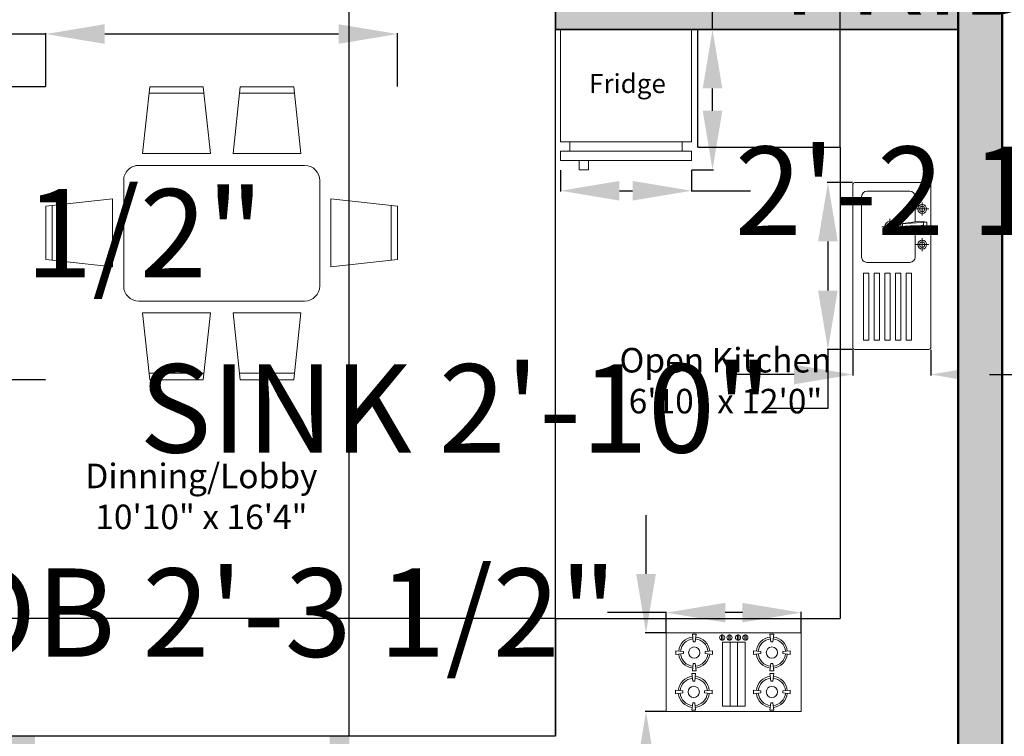
# Model space of a CAD drawing. Units: inches. Extents: x 2796 to 3603, y 978 to 1787.
# Tile 10 of 15: x 3224 to 3425, y 1312 to 1458. Entities that reach past the tile are written whole.
import ezdxf

# ---------------------------------------------------------------- set-up
doc = ezdxf.new("R2010")
doc.units = ezdxf.units.IN
for name, color, linetype, lineweight in [('A-ANNO-DIMS', 7, 'Continuous', 18), ('A-ANNO-TEXT', 7, 'Continuous', 18), ('A-AREA-IDEN', 7, 'Continuous', 18), ('A-EQPM', 3, 'Continuous', 18), ('A-FLOR-FIXT', 8, 'Continuous', 18), ('A-WALL-EXTR-PATT', 1, 'Continuous', 13), ('A-WALL-INTR-PATT', 5, 'Continuous', 13), ('Furniture', 2, 'Continuous', 18), ('Inner Wall', 5, 'Continuous', 35), ('Kitchen', 3, 'Continuous', 25), ('Outer Wall', 1, 'Continuous', 50)]:
    doc.layers.add(name, color=color, linetype=linetype, lineweight=lineweight)
doc.styles.get("Standard").update_dxf_attribs({"font": 'arial.ttf'})
doc.dimstyles.get("Standard").update_dxf_attribs({"dimtxt": 18, "dimasz": 12, "dimexe": 0.18, "dimexo": 0.0625, "dimgap": 0.09, "dimtad": 0, "dimtih": 1, "dimtoh": 1, "dimdec": 0, "dimzin": 0, "dimdsep": 46, "dimlunit": 3, "dimtxsty": 'Standard', "dimcen": 0.09, "dimadec": 0, "dimazin": 0, "dimtfac": 1, "dimtdec": 0, "dimtofl": 0, "dimtmove": 0, "dimatfit": 3, "dimfxl": 1, "dimtolj": 1, "dimtzin": 0, "dimarcsym": 0})

# ---------------------------------------------------------------- blocks, each defined once
blk = doc.blocks.new('A$C6D1B16CF')
for p, q in [((0.6411, 1.5), (0.6886, 1.9429)), ((0.684, 1.9), (1.0481, 1.9)), ((0.6886, 1.9429), (1.0435, 1.9429)), ((1.0435, 1.9429), (1.091, 1.5)), ((1.2411, 1.5), (1.2886, 1.9429)), ((1.284, 1.9), (1.6481, 1.9)), ((1.2886, 1.9429), (1.6435, 1.9429)), ((1.6435, 1.9429), (1.691, 1.5)), ((1.091, 1.5), (0.6411, 1.5)), ((1.691, 1.5), (1.2411, 1.5)), ((0.6161, 1.4214), (1.7161, 1.4214)), ((0.5161, 0.6214), (0.5161, 1.3214)), ((1.8161, 1.3214), (1.8161, 0.6214)), ((0, 1.1464), (0.4429, 1.1939)), ((0.4429, 1.1939), (0.4429, 0.744)), ((2.3321, 1.1464), (1.8892, 1.1939)), ((1.8892, 1.1939), (1.8892, 0.744)), ((0, 0.7916), (0, 1.1464)), ((0.0429, 0.787), (0.0429, 1.151)), ((2.2892, 0.787), (2.2892, 1.151)), ((2.3321, 0.7916), (2.3321, 1.1464)), ((0.4429, 0.744), (0, 0.7916)), ((1.8892, 0.744), (2.3321, 0.7916)), ((1.7161, 0.5214), (0.6161, 0.5214)), ((1.091, 0.4429), (0.6411, 0.4429)), ((0.6411, 0.4429), (0.6886, 0)), ((1.0435, 0), (1.091, 0.4429)), ((1.691, 0.4429), (1.2411, 0.4429)), ((1.2411, 0.4429), (1.2886, 0)), ((1.6435, 0), (1.691, 0.4429)), ((0.684, 0.0429), (1.0481, 0.0429)), ((0.6886, 0), (1.0435, 0)), ((1.284, 0.0429), (1.6481, 0.0429)), ((1.2886, 0), (1.6435, 0))]:
    blk.add_line(p, q)
for centre, start, end in [((0.6161, 1.3214), 90, 180), ((1.7161, 1.3214), 0, 90), ((0.6161, 0.6214), 180, 270), ((1.7161, 0.6214), 270, 0)]:
    blk.add_arc(centre, 0.1, start, end)
blk = doc.blocks.new('A$C57CF26DA')
for p, q in [((0, 0), (0, 420)), ((720, 420), (0, 420)), ((166.9, 413), (146.9, 413)), ((146.9, 413), (151.9, 373)), ((151.9, 373), (161.9, 373)), ((161.9, 373), (166.9, 413)), ((300, 390.9), (300, 49.1)), ((300, 390.9), (420, 390.9)), ((340, 390.9), (340, 49.1)), ((380, 390.9), (380, 49.1)), ((420, 390.9), (420, 49.1)), ((583.6, 413), (563.6, 413)), ((563.6, 413), (568.6, 373)), ((568.6, 373), (578.6, 373)), ((578.6, 373), (583.6, 413)), ((720, 0), (720, 420)), ((98.9, 320), (58.9, 325)), ((58.9, 325), (58.9, 305)), ((98.9, 310), (98.9, 320)), ((254.8, 325), (214.8, 320)), ((214.8, 320), (214.8, 310)), ((254.8, 305), (254.8, 325)), ((515.6, 320), (475.6, 325)), ((475.6, 325), (475.6, 305)), ((515.6, 310), (515.6, 320)), ((671.6, 325), (631.6, 320)), ((631.6, 320), (631.6, 310)), ((671.6, 305), (671.6, 325)), ((58.9, 305), (98.9, 310)), ((214.8, 310), (254.8, 305)), ((475.6, 305), (515.6, 310)), ((631.6, 310), (671.6, 305)), ((151.9, 257), (146.9, 217)), ((146.9, 217), (166.9, 217)), ((161.9, 257), (151.9, 257)), ((166.9, 217), (161.9, 257)), ((568.6, 257), (563.6, 217)), ((563.6, 217), (583.6, 217)), ((578.6, 257), (568.6, 257)), ((583.6, 217), (578.6, 257)), ((166.9, 203), (146.9, 203)), ((146.9, 203), (151.9, 163)), ((151.9, 163), (161.9, 163)), ((161.9, 163), (166.9, 203)), ((581.1, 203), (561.1, 203)), ((561.1, 203), (566.1, 163)), ((566.1, 163), (576.1, 163)), ((576.1, 163), (581.1, 203)), ((98.9, 110), (58.9, 115)), ((58.9, 115), (58.9, 95)), ((98.9, 100), (98.9, 110)), ((254.8, 115), (214.8, 110)), ((214.8, 110), (214.8, 100)), ((254.8, 95), (254.8, 115)), ((513.1, 110), (473.1, 115)), ((473.1, 115), (473.1, 95)), ((513.1, 100), (513.1, 110)), ((669, 115), (629, 110)), ((629, 110), (629, 100)), ((669, 95), (669, 115)), ((58.9, 95), (98.9, 100)), ((214.8, 100), (254.8, 95)), ((473.1, 95), (513.1, 100)), ((629, 100), (669, 95)), ((151.9, 47), (146.9, 7)), ((146.9, 7), (166.9, 7)), ((161.9, 47), (151.9, 47)), ((166.9, 7), (161.9, 47)), ((301.5, 38.7), (294.7, 38.7)), ((294.7, 38.7), (294.7, 11.3)), ((294.7, 11.3), (301.5, 11.3)), ((420, 49.1), (300, 49.1)), ((301.5, 11.3), (301.5, 38.7)), ((340.5, 38.7), (333.7, 38.7)), ((333.7, 38.7), (333.7, 11.3)), ((333.7, 11.3), (340.5, 11.3)), ((340.5, 11.3), (340.5, 38.7)), ((379.7, 11.3), (379.7, 38.7)), ((379.7, 38.7), (386.5, 38.7)), ((386.5, 11.3), (379.7, 11.3)), ((386.5, 38.7), (386.5, 11.3)), ((418.7, 11.3), (418.7, 38.7)), ((418.7, 38.7), (425.5, 38.7)), ((425.5, 11.3), (418.7, 11.3)), ((425.5, 38.7), (425.5, 11.3)), ((566.1, 47), (561.1, 7)), ((561.1, 7), (581.1, 7)), ((576.1, 47), (566.1, 47)), ((581.1, 7), (576.1, 47)), ((720, 0), (0, 0))]:
    blk.add_line(p, q)
for centre in [(156.9, 315), (573.6, 315), (156.9, 105), (571.1, 105)]:
    blk.add_circle(centre, 30)
for centre, radius, start, end in [((156.9, 315), 83, 95.5849, 174.4151), ((156.9, 315), 73, 95.3738, 174.6262), ((156.9, 315), 73, 5.3738, 84.6262), ((156.9, 315), 83, 5.5849, 84.4151), ((573.6, 315), 83, 95.5849, 174.4151), ((573.6, 315), 73, 95.3738, 174.6262), ((573.6, 315), 73, 5.3738, 84.6262), ((573.6, 315), 83, 5.5849, 84.4151), ((156.9, 315), 83, 185.5849, 264.4151), ((156.9, 315), 73, 185.3738, 264.6262), ((156.9, 315), 73, 275.3738, 354.6262), ((156.9, 315), 83, 275.5849, 354.4151), ((573.6, 315), 83, 185.5849, 264.4151), ((573.6, 315), 73, 185.3738, 264.6262), ((573.6, 315), 73, 275.3738, 354.6262), ((573.6, 315), 83, 275.5849, 354.4151), ((156.9, 105), 83, 95.5849, 174.4151), ((156.9, 105), 73, 95.3738, 174.6262), ((156.9, 105), 73, 5.3738, 84.6262), ((156.9, 105), 83, 5.5849, 84.4151), ((571.1, 105), 83, 95.5849, 174.4151), ((571.1, 105), 73, 95.3738, 174.6262), ((571.1, 105), 73, 5.3738, 84.6262), ((571.1, 105), 83, 5.5849, 84.4151), ((156.9, 105), 83, 185.5849, 264.4151), ((156.9, 105), 73, 185.3738, 264.6262), ((156.9, 105), 73, 275.3738, 354.6262), ((156.9, 105), 83, 275.5849, 354.4151), ((571.1, 105), 83, 185.5849, 264.4151), ((571.1, 105), 73, 185.3738, 264.6262), ((571.1, 105), 73, 275.3738, 354.6262), ((571.1, 105), 83, 275.5849, 354.4151), ((298.1, 25), 13.7, 104.4775, 255.5225), ((298.1, 25), 13.7, 284.4775, 75.5225), ((337.1, 25), 13.7, 104.4775, 255.5225), ((337.1, 25), 13.7, 284.4775, 75.5225), ((383.1, 25), 13.7, 104.4775, 255.5225), ((383.1, 25), 13.7, 284.4775, 75.5225), ((422.1, 25), 13.7, 104.4775, 255.5225), ((422.1, 25), 13.7, 284.4775, 75.5225)]:
    blk.add_arc(centre, radius, start, end)
blk = doc.blocks.new('A$C7C492201')
for p, q in [((0, 10), (0, 426.6)), ((10, 436.6), (927.3, 436.6)), ((111.9, 388.7), (185, 388.7)), ((148.5, 425.2), (148.5, 352.2)), ((223.5, 415), (217, 376.2)), ((223.5, 415), (231.8, 268.5)), ((223.5, 415), (248.5, 415)), ((224.6, 395.4), (248.5, 395.4)), ((273.5, 415), (248.5, 415)), ((272.3, 395.4), (248.5, 395.4)), ((273.5, 415), (265.2, 268.5)), ((273.5, 415), (279.9, 376.2)), ((311.9, 388.7), (385, 388.7)), ((348.5, 425.2), (348.5, 352.2)), ((937.3, 10), (937.3, 426.6)), ((220.8, 348.8), (78.5, 348.8)), ((217, 376.2), (231.8, 268.5)), ((279.9, 376.2), (265.2, 268.5)), ((418.5, 348.8), (276.2, 348.8)), ((48.5, 318.8), (48.5, 78.8)), ((231.3, 278.6), (248.5, 278.6)), ((265.6, 278.6), (248.5, 278.6)), ((448.5, 318.8), (448.5, 78.8)), ((509.1, 328.4), (509.1, 298.4)), ((509.1, 328.4), (885, 328.4)), ((509.1, 298.4), (885, 298.4)), ((885, 328.4), (885, 298.4)), ((231.8, 268.5), (248.5, 268.5)), ((265.2, 268.5), (248.5, 268.5)), ((248.5, 252.8), (248.5, 162.6)), ((509.1, 268.4), (509.1, 238.4)), ((509.1, 268.4), (885, 268.4)), ((509.1, 238.4), (885, 238.4)), ((885, 268.4), (885, 238.4)), ((203.4, 207.7), (293.5, 207.7)), ((509.1, 208.4), (885, 208.4)), ((509.1, 208.4), (509.1, 178.4)), ((509.1, 178.4), (885, 178.4)), ((885, 208.4), (885, 178.4)), ((509.1, 148.4), (509.1, 118.4)), ((509.1, 148.4), (885, 148.4)), ((509.1, 118.4), (885, 118.4)), ((885, 148.4), (885, 118.4)), ((509.1, 88.4), (509.1, 58.4)), ((509.1, 88.4), (885, 88.4)), ((509.1, 58.4), (885, 58.4)), ((885, 88.4), (885, 58.4)), ((927.3, 0), (10, 0)), ((418.5, 48.8), (78.5, 48.8))]:
    blk.add_line(p, q)
for centre, radius in [((148.5, 388.7), 25), ((148.5, 388.7), 15), ((348.5, 388.7), 25), ((348.5, 388.7), 15), ((248.5, 207.7), 30), ((248.5, 207.7), 20)]:
    blk.add_circle(centre, radius)
for centre, radius, start, end in [((10, 426.6), 10, 90, 180), ((247.3, 388), 7.19, 80.5252, 279.4748), ((249.6, 388), 7.19, 260.5252, 99.4748), ((927.3, 426.6), 10, 0, 90), ((78.5, 318.8), 30, 90, 180), ((418.5, 318.8), 30, 0, 90), ((78.5, 78.8), 30, 180, 270), ((418.5, 78.8), 30, 270, 0), ((10, 10), 10, 180, 270), ((927.3, 10), 10, 270, 0)]:
    blk.add_arc(centre, radius, start, end)
blk = doc.blocks.new('REFRI-00')
for points in [[(-0.35, 0.35), (-0.35, -0.25), (0.35, -0.25), (0.35, 0.35), (-0.35, 0.35)], [(-0.3, -0.3), (-0.3, -0.25)], [(0.3, -0.3), (0.3, -0.25)], [(-0.35, -0.3), (-0.35, -0.35), (0.35, -0.35), (0.35, -0.3), (-0.35, -0.3)], [(-0.25, -0.35), (-0.25, -0.4), (-0.2, -0.4), (-0.2, -0.35)]]:
    blk.add_lwpolyline(points)
blk = doc.blocks.new('*D32')
at = {"layer": 'A-ANNO-DIMS', "color": 0, "lineweight": -2, "transparency": 16777216}
for p, q in [((3229.46, 1454.75), (3217.46, 1454.75)), ((3229.46, 1444.07), (3229.46, 1454.93)), ((3289.09, 1454.75), (3241.46, 1454.75)), ((3301.09, 1444.07), (3301.09, 1454.93))]:
    blk.add_line(p, q, dxfattribs=at)
at = {"layer": 'A-ANNO-DIMS', "color": 0, "transparency": 16777216}
for points in [[(3241.46, 1456.75), (3241.46, 1452.75), (3229.46, 1454.75)], [(3289.09, 1456.75), (3289.09, 1452.75), (3301.09, 1454.75)]]:
    blk.add_solid(points, dxfattribs=at)
at = {"layer": 'Defpoints', "color": 0, "transparency": 16777216}
for p in [(3229.46, 1454.75), (3229.46, 1444.01), (3301.09, 1444.01)]:
    blk.add_point(p, dxfattribs=at)
at = {"layer": 'A-ANNO-DIMS', "color": 0, "transparency": 16777216, "insert": (3090.48, 1454.75), "char_height": 18, "attachment_point": 5}
blk.add_mtext('\\A1;DINING SET 5\'-11 1/2"', dxfattribs=at)
blk = doc.blocks.new('*D33')
at = {"layer": 'A-ANNO-DIMS', "color": 0, "lineweight": -2, "transparency": 16777216}
for p, q in [((3229.39, 1444.01), (3218.53, 1444.01)), ((3218.71, 1432.01), (3218.71, 1423.57)), ((3218.71, 1396.33), (3218.71, 1404.77)), ((3229.39, 1384.33), (3218.53, 1384.33))]:
    blk.add_line(p, q, dxfattribs=at)
at = {"layer": 'A-ANNO-DIMS', "color": 0, "transparency": 16777216}
for points in [[(3216.71, 1432.01), (3220.71, 1432.01), (3218.71, 1444.01)], [(3216.71, 1396.33), (3220.71, 1396.33), (3218.71, 1384.33)]]:
    blk.add_solid(points, dxfattribs=at)
at = {"layer": 'Defpoints', "color": 0, "transparency": 16777216}
for p in [(3229.46, 1444.01), (3218.71, 1384.33), (3229.46, 1384.33)]:
    blk.add_point(p, dxfattribs=at)
at = {"layer": 'A-ANNO-DIMS', "color": 0, "transparency": 16777216, "insert": (3218.71, 1414.17), "char_height": 18, "attachment_point": 5}
blk.add_mtext('\\A1;4\'-11 1/2"', dxfattribs=at)
blk = doc.blocks.new('*D34')
at = {"layer": 'A-ANNO-DIMS', "color": 0, "lineweight": -2, "transparency": 16777216}
for p, q in [((3355.83, 1336.87), (3343.83, 1336.87)), ((3355.83, 1332.81), (3355.83, 1337.05)), ((3371.32, 1336.87), (3367.83, 1336.87)), ((3383.32, 1332.81), (3383.32, 1337.05))]:
    blk.add_line(p, q, dxfattribs=at)
at = {"layer": 'A-ANNO-DIMS', "color": 0, "transparency": 16777216}
for points in [[(3367.83, 1338.87), (3367.83, 1334.87), (3355.83, 1336.87)], [(3371.32, 1338.87), (3371.32, 1334.87), (3383.32, 1336.87)]]:
    blk.add_solid(points, dxfattribs=at)
at = {"layer": 'Defpoints', "color": 0, "transparency": 16777216}
for p in [(3355.83, 1336.87), (3355.83, 1332.75), (3383.32, 1332.75)]:
    blk.add_point(p, dxfattribs=at)
at = {"layer": 'A-ANNO-DIMS', "color": 0, "transparency": 16777216, "insert": (3268.59, 1336.87), "char_height": 18, "attachment_point": 5}
blk.add_mtext('\\A1;HOB 2\'-3 1/2"', dxfattribs=at)
blk = doc.blocks.new('*D35')
at = {"layer": 'A-ANNO-DIMS', "color": 0, "lineweight": -2, "transparency": 16777216}
for p, q in [((3351.71, 1344.75), (3351.71, 1356.75)), ((3355.77, 1332.75), (3351.53, 1332.75)), ((3355.77, 1316.72), (3351.53, 1316.72)), ((3351.71, 1304.72), (3351.71, 1292.72)), ((3351.71, 1292.72), (3339.71, 1292.72))]:
    blk.add_line(p, q, dxfattribs=at)
at = {"layer": 'A-ANNO-DIMS', "color": 0, "transparency": 16777216}
for points in [[(3349.71, 1344.75), (3353.71, 1344.75), (3351.71, 1332.75)], [(3349.71, 1304.72), (3353.71, 1304.72), (3351.71, 1316.72)]]:
    blk.add_solid(points, dxfattribs=at)
at = {"layer": 'Defpoints', "color": 0, "transparency": 16777216}
for p in [(3355.83, 1332.75), (3351.71, 1316.72), (3355.83, 1316.72)]:
    blk.add_point(p, dxfattribs=at)
at = {"layer": 'A-ANNO-DIMS', "color": 0, "transparency": 16777216, "insert": (3316.54, 1292.72), "char_height": 18, "attachment_point": 5}
blk.add_mtext('\\A1;1\'-4"', dxfattribs=at)
blk = doc.blocks.new('*D36')
at = {"layer": 'A-ANNO-DIMS', "color": 0, "lineweight": -2, "transparency": 16777216}
for p, q in [((3393.79, 1424.5), (3388.57, 1424.5)), ((3388.75, 1412.5), (3388.75, 1402.49)), ((3393.79, 1390.49), (3388.57, 1390.49)), ((3388.75, 1390.49), (3388.75, 1378.49)), ((3388.75, 1378.49), (3376.75, 1378.49))]:
    blk.add_line(p, q, dxfattribs=at)
at = {"layer": 'A-ANNO-DIMS', "color": 0, "transparency": 16777216}
for points in [[(3386.75, 1412.5), (3390.75, 1412.5), (3388.75, 1424.5)], [(3386.75, 1402.49), (3390.75, 1402.49), (3388.75, 1390.49)]]:
    blk.add_solid(points, dxfattribs=at)
at = {"layer": 'Defpoints', "color": 0, "transparency": 16777216}
for p in [(3393.85, 1424.5), (3388.75, 1390.49), (3393.85, 1390.49)]:
    blk.add_point(p, dxfattribs=at)
at = {"layer": 'A-ANNO-DIMS', "color": 0, "transparency": 16777216, "insert": (3312.95, 1378.49), "char_height": 18, "attachment_point": 5}
blk.add_mtext('\\A1;SINK 2\'-10"', dxfattribs=at)
blk = doc.blocks.new('*D37')
at = {"layer": 'A-ANNO-DIMS', "color": 0, "lineweight": -2, "transparency": 16777216}
for p, q in [((3393.85, 1390.43), (3393.85, 1385.21)), ((3409.69, 1390.43), (3409.69, 1385.21)), ((3381.85, 1385.39), (3369.85, 1385.39)), ((3421.69, 1385.39), (3433.69, 1385.39))]:
    blk.add_line(p, q, dxfattribs=at)
at = {"layer": 'A-ANNO-DIMS', "color": 0, "transparency": 16777216}
for points in [[(3381.85, 1387.39), (3381.85, 1383.39), (3393.85, 1385.39)], [(3421.69, 1387.39), (3421.69, 1383.39), (3409.69, 1385.39)]]:
    blk.add_solid(points, dxfattribs=at)
at = {"layer": 'Defpoints', "color": 0, "transparency": 16777216}
for p in [(3393.85, 1390.49), (3409.69, 1390.49), (3409.69, 1385.39)]:
    blk.add_point(p, dxfattribs=at)
at = {"layer": 'A-ANNO-DIMS', "color": 0, "transparency": 16777216, "insert": (3456.86, 1385.39), "char_height": 18, "attachment_point": 5}
blk.add_mtext('\\A1;1\'-4"', dxfattribs=at)
blk = doc.blocks.new('*D38')
at = {"layer": 'A-ANNO-DIMS', "color": 0, "lineweight": -2, "transparency": 16777216}
for p, q in [((3365.25, 1455.68), (3365.25, 1467.68)), ((3365.25, 1467.68), (3377.25, 1467.68)), ((3361.02, 1455.68), (3365.43, 1455.68)), ((3365.25, 1439.11), (3365.25, 1443.68)), ((3361.02, 1427.11), (3365.43, 1427.11))]:
    blk.add_line(p, q, dxfattribs=at)
at = {"layer": 'A-ANNO-DIMS', "color": 0, "transparency": 16777216}
for points in [[(3363.25, 1443.68), (3367.25, 1443.68), (3365.25, 1455.68)], [(3363.25, 1439.11), (3367.25, 1439.11), (3365.25, 1427.11)]]:
    blk.add_solid(points, dxfattribs=at)
at = {"layer": 'Defpoints', "color": 0, "transparency": 16777216}
for p in [(3360.96, 1455.68), (3365.25, 1455.68), (3360.96, 1427.11)]:
    blk.add_point(p, dxfattribs=at)
at = {"layer": 'A-ANNO-DIMS', "color": 0, "transparency": 16777216, "insert": (3472.71, 1467.68), "char_height": 18, "attachment_point": 5}
blk.add_mtext('\\A1;FRIDGE 2\'-4 1/2"', dxfattribs=at)
blk = doc.blocks.new('*D39')
at = {"layer": 'A-ANNO-DIMS', "color": 0, "lineweight": -2, "transparency": 16777216}
for p, q in [((3334.3, 1427.04), (3334.3, 1422.64)), ((3360.96, 1427.04), (3360.96, 1422.64)), ((3346.3, 1422.82), (3348.96, 1422.82)), ((3360.96, 1422.82), (3372.96, 1422.82))]:
    blk.add_line(p, q, dxfattribs=at)
at = {"layer": 'A-ANNO-DIMS', "color": 0, "transparency": 16777216}
for points in [[(3346.3, 1424.82), (3346.3, 1420.82), (3334.3, 1422.82)], [(3348.96, 1424.82), (3348.96, 1420.82), (3360.96, 1422.82)]]:
    blk.add_solid(points, dxfattribs=at)
at = {"layer": 'Defpoints', "color": 0, "transparency": 16777216}
for p in [(3334.3, 1427.11), (3360.96, 1427.11), (3360.96, 1422.82)]:
    blk.add_point(p, dxfattribs=at)
at = {"layer": 'A-ANNO-DIMS', "color": 0, "transparency": 16777216, "insert": (3418.1, 1422.82), "char_height": 18, "attachment_point": 5}
blk.add_mtext('\\A1;2\'-2 1/2"', dxfattribs=at)
blk = doc.blocks.new('*D42')
at = {"layer": 'A-ANNO-DIMS', "color": 0, "lineweight": -2, "transparency": 16777216}
for p, q in [((3291.25, 1311.74), (3291.25, 1775.56)), ((3303.25, 1775.38), (3321.25, 1775.38)), ((3333.25, 1311.74), (3333.25, 1775.56)), ((3333.25, 1775.38), (3345.25, 1775.38))]:
    blk.add_line(p, q, dxfattribs=at)
at = {"layer": 'A-ANNO-DIMS', "color": 0, "transparency": 16777216}
for points in [[(3303.25, 1777.38), (3303.25, 1773.38), (3291.25, 1775.38)], [(3321.25, 1777.38), (3321.25, 1773.38), (3333.25, 1775.38)]]:
    blk.add_solid(points, dxfattribs=at)
at = {"layer": 'Defpoints', "color": 0, "transparency": 16777216}
for p in [(3333.25, 1775.38), (3291.25, 1311.68), (3333.25, 1311.68)]:
    blk.add_point(p, dxfattribs=at)
at = {"layer": 'A-ANNO-DIMS', "color": 0, "transparency": 16777216, "insert": (3369.25, 1775.38), "char_height": 18, "attachment_point": 5}
blk.add_mtext('\\A1;3\'-6"', dxfattribs=at)
blk = doc.blocks.new('*D53')
at = {"layer": 'A-ANNO-DIMS', "color": 0, "lineweight": -2, "transparency": 16777216}
for p, q in [((3031.545499, 1347.67534), (3031.545499, 1359.67534)), ((3333.182999, 1335.67534), (3031.365499, 1335.67534)), ((3333.182999, 1311.67534), (3031.365499, 1311.67534)), ((3031.545499, 1299.67534), (3031.545499, 1287.67534))]:
    blk.add_line(p, q, dxfattribs=at)
at = {"layer": 'A-ANNO-DIMS', "color": 0, "transparency": 16777216}
for points in [[(3029.545499, 1347.67534), (3033.545499, 1347.67534), (3031.545499, 1335.67534)], [(3029.545499, 1299.67534), (3033.545499, 1299.67534), (3031.545499, 1311.67534)]]:
    blk.add_solid(points, dxfattribs=at)
at = {"layer": 'Defpoints', "color": 0, "transparency": 16777216}
for p in [(3031.545499, 1335.67534), (3333.245499, 1335.67534), (3333.245499, 1311.67534)]:
    blk.add_point(p, dxfattribs=at)
at = {"layer": 'A-ANNO-DIMS', "color": 0, "transparency": 16777216, "insert": (3031.545499, 1323.67534), "char_height": 18, "attachment_point": 5}
blk.add_mtext('\\A1;2\'-0"', dxfattribs=at)
blk = doc.blocks.new('*D54')
at = {"layer": 'A-ANNO-DIMS', "color": 0, "lineweight": -2, "transparency": 16777216}
for p, q in [((3379.25, 1775.38), (3367.25, 1775.38)), ((3391.25, 1431.74), (3391.25, 1775.56)), ((3415.25, 1455.74), (3415.25, 1775.56)), ((3427.25, 1775.38), (3439.25, 1775.38))]:
    blk.add_line(p, q, dxfattribs=at)
at = {"layer": 'A-ANNO-DIMS', "color": 0, "transparency": 16777216}
for points in [[(3379.25, 1777.38), (3379.25, 1773.38), (3391.25, 1775.38)], [(3427.25, 1777.38), (3427.25, 1773.38), (3415.25, 1775.38)]]:
    blk.add_solid(points, dxfattribs=at)
at = {"layer": 'Defpoints', "color": 0, "transparency": 16777216}
for p in [(3415.25, 1775.38), (3415.25, 1455.68), (3391.25, 1431.68)]:
    blk.add_point(p, dxfattribs=at)
at = {"layer": 'A-ANNO-DIMS', "color": 0, "transparency": 16777216, "insert": (3463.41, 1775.38), "char_height": 18, "attachment_point": 5}
blk.add_mtext('\\A1;2\'-0"', dxfattribs=at)

msp = doc.modelspace()

# ---------------------------------------------------------------- hatches: boundary and pattern name
at = {"layer": 'A-WALL-EXTR-PATT'}
h = msp.add_hatch(color=256, dxfattribs=at)
h.dxf.hatch_style = 1
h.paths.add_polyline_path([(3424.25, 1736.68), (3070.25, 1736.68), (3070.25, 1106.68), (3227.25, 1106.68), (3227.25, 1115.68), (3226.75, 1115.68), (3223.75, 1115.68), (3079.25, 1115.68), (3079.25, 1727.68), (3127.25, 1727.68), (3415.25, 1727.68), (3415.25, 1188.68), (3424.25, 1188.68)])
h.paths.add_polyline_path([(3291.25, 1032.68), (3074.25, 1032.68), (3074.25, 1106.68), (3070.25, 1106.68), (3070.25, 1028.68), (3291.25, 1028.68)])
h.paths.add_polyline_path([(3291.25, 1115.68), (3281.25, 1115.68), (3281.25, 1106.68), (3291.25, 1106.68)], flags=17)
h.paths.add_polyline_path([(3301.25, 1037.68), (3291.25, 1037.68), (3291.25, 1028.68), (3301.25, 1028.68)])
h.paths.add_polyline_path([(3424.25, 1037.68), (3414.25, 1037.68), (3414.25, 1028.68), (3424.25, 1028.68)])
h.paths.add_polyline_path([(3424.25, 1188.68), (3420.25, 1188.68), (3420.25, 1037.68), (3424.25, 1037.68)])
at = {"layer": 'A-WALL-INTR-PATT'}
h = msp.add_hatch(color=256, dxfattribs=at)
h.dxf.hatch_style = 1
h.paths.add_polyline_path([(3249.25, 1727.68), (3245.25, 1727.68), (3245.25, 1655.68), (3103.25, 1655.68), (3103.25, 1651.68), (3245.25, 1651.68), (3245.25, 1503.68), (3249.25, 1503.68)])
h.paths.add_polyline_path([(3131.25, 1727.68), (3127.25, 1727.68), (3127.25, 1703.68), (3127.25, 1679.68), (3131.25, 1679.68)], flags=17)
h.paths.add_polyline_path([(3391.25, 1655.68), (3325.25, 1655.68), (3325.25, 1727.68), (3321.25, 1727.68), (3321.25, 1655.68), (3273.25, 1655.68), (3273.25, 1651.68), (3391.25, 1651.68)])
h.paths.add_polyline_path([(3203.25, 1459.68), (3079.25, 1459.68), (3079.25, 1455.68), (3199.25, 1455.68), (3199.25, 1431.68), (3199.25, 1347.68), (3203.25, 1347.68)])
h.paths.add_polyline_path([(3209.25, 1507.68), (3079.25, 1507.68), (3079.25, 1503.68), (3209.25, 1503.68)])
h.paths.add_polyline_path([(3415.25, 1507.68), (3285.25, 1507.68), (3285.25, 1503.68), (3415.25, 1503.68)])
h.paths.add_polyline_path([(3415.25, 1459.68), (3333.25, 1459.68), (3333.25, 1455.68), (3415.25, 1455.68)])
h.paths.add_polyline_path([(3291.25, 1311.68), (3287.25, 1311.68), (3287.25, 1192.68), (3227.25, 1192.68), (3227.25, 1267.68), (3263.25, 1267.68), (3263.25, 1271.68), (3223.25, 1271.68), (3223.25, 1151.68), (3227.25, 1151.68), (3227.25, 1188.68), (3291.25, 1188.68)])
h.paths.add_polyline_path([(3227.25, 1311.68), (3079.25, 1311.68), (3079.25, 1307.68), (3227.25, 1307.68)])

# ---------------------------------------------------------------- linework, layer by layer
at = {"layer": 'Inner Wall'}
for q in [(3333.25, 1459.68), (3415.25, 1455.68)]:
    msp.add_line((3333.25, 1455.68), q, dxfattribs=at)
at = {"layer": 'Kitchen'}
for p, q in [((3333.25, 1455.68), (3415.25, 1455.68)), ((3362.25, 1431.68), (3362.25, 1455.68)), ((3415.25, 1455.68), (3415.25, 1311.68)), ((3362.25, 1431.68), (3391.25, 1431.68)), ((3391.25, 1431.68), (3391.25, 1335.68)), ((3333.25, 1335.68), (3391.25, 1335.68)), ((3333.25, 1335.68), (3333.25, 1311.68))]:
    msp.add_line(p, q, dxfattribs=at)
at = {"layer": 'Outer Wall'}
for p, q in [((3424.25, 1736.68), (3424.25, 1028.68)), ((3415.25, 1727.68), (3415.25, 1188.68))]:
    msp.add_line(p, q, dxfattribs=at)

# ---------------------------------------------------------------- block references
at = {"layer": 'A-EQPM', "xscale": 38.0932829071003, "yscale": 38.0932829071003, "zscale": 38.0932829071003}
msp.add_blockref('REFRI-00', (3347.63, 1442.34), dxfattribs=at)
at = {"layer": 'A-EQPM', "xscale": 0.0381707681172169, "yscale": 0.0381707681172169, "zscale": 0.0381707681172169, "rotation": 180}
msp.add_blockref('A$C57CF26DA', (3383.32, 1332.75), dxfattribs=at)
at = {"layer": 'A-FLOR-FIXT', "xscale": 0.0362851414289068, "yscale": 0.0362851414289068, "zscale": 0.0362851414289068, "rotation": 270}
msp.add_blockref('A$C7C492201', (3393.85, 1424.5), dxfattribs=at)
at = {"layer": 'Furniture', "xscale": 30.71454900626152, "yscale": 30.71454900626152, "zscale": 30.71454900626152, "rotation": 180}
msp.add_blockref('A$C6D1B16CF', (3301.09, 1444.01), dxfattribs=at)

# ---------------------------------------------------------------- texts
at = {"layer": 'A-ANNO-TEXT', "insert": (3338.95, 1446.6), "char_height": 3.878, "attachment_point": 1}
msp.add_mtext_dynamic_manual_height_columns('\\pxqc;{\\fTimes New Roman|b0|i0|c0|p18;Fridge}', width=17.9518, gutter_width=4.85, heights=[0], dxfattribs=at)
at = {"layer": 'A-AREA-IDEN', "char_height": 5, "attachment_point": 3}
for s, insert in [('\\pxqc;{\\fTimes New Roman|b0|i0|c0|p18;Open Kitchen\\P6\'10" x 12\'0"}', (3395.64, 1390.8)), ('\\pxqc;{\\fTimes New Roman|b0|i0|c0|p18;Dinning/Lobby\\P10\'10" x 16\'4"}', (3288.89, 1367.22))]:
    msp.add_mtext_dynamic_manual_height_columns(s, width=55.5021, gutter_width=12.5, heights=[0], dxfattribs=dict(at, insert=insert))

# ---------------------------------------------------------------- dimensions: what is measured, and where the dimension line sits
at = {"layer": 'A-ANNO-DIMS'}
for base, p1, p2, picture, middle in [((3333.25, 1775.38), (3291.25, 1311.68), (3333.25, 1311.68), '*D42', (3369.25, 1775.38)), ((3415.25, 1775.38), (3391.25, 1431.68), (3415.25, 1455.68), '*D54', (3463.41, 1775.38)), ((3360.96, 1422.82), (3334.3, 1427.11), (3360.96, 1427.11), '*D39', (3418.1, 1422.82)), ((3409.69, 1385.39), (3393.85, 1390.49), (3409.69, 1390.49), '*D37', (3456.86, 1385.39))]:
    dim = msp.add_linear_dim(base=base, p1=p1, p2=p2, dimstyle='Standard', override={"dimdec": 1, "dimlfac": 1, "dimrnd": 0, "dimzin": 1, "dimdsep": 46, "dimlunit": 4, "dimfrac": 2}, dxfattribs=at)
    dim.commit()
    dim.dimension.update_dxf_attribs({"geometry": picture, "text_midpoint": middle})
for base, p1, p2, angle, text, picture, middle in [((3229.46, 1454.75), (3301.09, 1444.01), (3229.46, 1444.01), 180, 'DINING SET <>', '*D32', (3090.48, 1454.75)), ((3365.25, 1455.68), (3360.96, 1427.11), (3360.96, 1455.68), 90, 'FRIDGE <>', '*D38', (3472.71, 1467.68)), ((3388.75, 1390.49), (3393.85, 1424.5), (3393.85, 1390.49), 270, 'SINK <>', '*D36', (3312.95, 1378.49)), ((3355.83, 1336.87), (3383.32, 1332.75), (3355.83, 1332.75), 180, 'HOB <>', '*D34', (3268.59, 1336.87))]:
    dim = msp.add_linear_dim(base=base, p1=p1, p2=p2, angle=angle, text=text, dimstyle='Standard', override={"dimdec": 1, "dimlfac": 1, "dimrnd": 0, "dimzin": 1, "dimdsep": 46, "dimlunit": 4, "dimfrac": 2}, dxfattribs=at)
    dim.commit()
    dim.dimension.update_dxf_attribs({"geometry": picture, "text_midpoint": middle})
for base, p1, p2, angle, picture, middle in [((3218.71, 1384.33), (3229.46, 1444.01), (3229.46, 1384.33), 270, '*D33', (3218.71, 1414.17)), ((3031.55, 1335.68), (3333.25, 1311.68), (3333.25, 1335.68), 90, '*D53', (3031.55, 1323.68)), ((3351.71, 1316.72), (3355.83, 1332.75), (3355.83, 1316.72), 270, '*D35', (3316.54, 1292.72))]:
    dim = msp.add_linear_dim(base=base, p1=p1, p2=p2, angle=angle, dimstyle='Standard', override={"dimdec": 1, "dimlfac": 1, "dimrnd": 0, "dimzin": 1, "dimdsep": 46, "dimlunit": 4, "dimfrac": 2}, dxfattribs=at)
    dim.commit()
    dim.dimension.update_dxf_attribs({"geometry": picture, "text_midpoint": middle})

doc.saveas('drawing.dxf')
